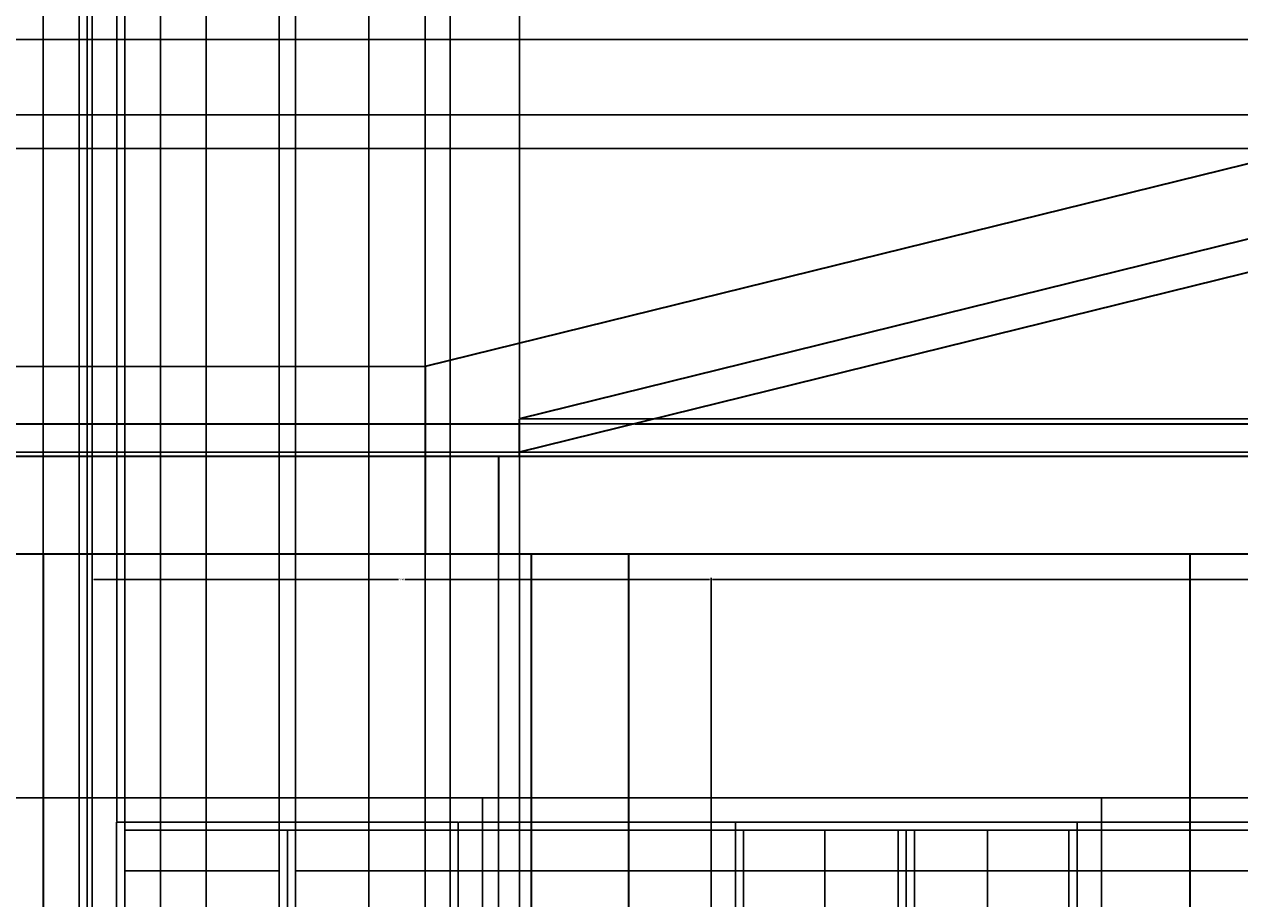
# Model space of a CAD drawing. Units: inches. Extents: x 2154 to 2740, y 571 to 1084.
# Tile 4 of 13: x 2235 to 2384, y 861 to 969. Entities that reach past the tile are written whole.
import ezdxf

# ---------------------------------------------------------------- set-up
doc = ezdxf.new("R2010")
doc.units = ezdxf.units.IN
for name, color, linetype, lineweight in [('A-ANNO-DIMS', 2, 'Continuous', 18), ('A-ELEV', 7, 'Continuous', 35), ('A-GLAZ', 4, 'Continuous', 25), ('A-ROOF', 1, 'Continuous', 35)]:
    doc.layers.add(name, color=color, linetype=linetype, lineweight=lineweight)
doc.styles.get("Standard").update_dxf_attribs({"font": 'arial.ttf'})
doc.dimstyles.get("Standard").update_dxf_attribs({"dimtxt": 0.18, "dimasz": 0.18, "dimexe": 0.18, "dimexo": 0.0625, "dimgap": 0.09, "dimtad": 0, "dimtih": 1, "dimtoh": 1, "dimdec": 4, "dimzin": 0, "dimdsep": 46, "dimtxsty": 'Standard', "dimcen": 0.09, "dimadec": 0, "dimazin": 0, "dimtfac": 1, "dimtdec": 4, "dimtofl": 0, "dimtmove": 0, "dimatfit": 3, "dimfxl": 1, "dimtolj": 1, "dimtzin": 0, "dimarcsym": 0})

# ---------------------------------------------------------------- blocks, each defined once
blk = doc.blocks.new('WIN-ELEV-1200')
for p, q in [((0, 50), (48, 50)), ((0, 0), (0, 50)), ((48, 0), (48, 50)), ((3, 0), (3, 47)), ((3, 47), (45, 47)), ((45, 0), (45, 47)), ((4, 46), (44, 46)), ((4, 0), (4, 46)), ((14, 0), (14, 46)), ((23, 0), (23, 46)), ((24, 0), (24, 46)), ((25, 0), (25, 46)), ((34, 0), (34, 46)), ((44, 0), (44, 46)), ((4, 41), (23, 41)), ((25, 41), (44, 41)), ((4, 32), (23, 32)), ((25, 32), (44, 32)), ((4, 23), (23, 23)), ((25, 23), (44, 23)), ((4, 14), (23, 14)), ((25, 14), (44, 14)), ((4, 5), (23, 5)), ((25, 5), (44, 5))]:
    blk.add_line(p, q)
blk = doc.blocks.new('*D8')
at = {"layer": 'A-ANNO-DIMS', "color": 0, "lineweight": -2, "transparency": 16777216}
for p, q in [((2284.21, 926.63), (2284.21, 953.59)), ((2601.21, 926.54), (2601.21, 953.51)), ((2284.39, 953.41), (2442.43, 953.37)), ((2601.03, 953.33), (2443, 953.37))]:
    blk.add_line(p, q, dxfattribs=at)
at = {"layer": 'A-ANNO-DIMS', "color": 0, "transparency": 16777216}
for points in [[(2284.39, 953.44), (2284.39, 953.38), (2284.21, 953.41)], [(2601.03, 953.36), (2601.03, 953.3), (2601.21, 953.33)]]:
    blk.add_solid(points, dxfattribs=at)
at = {"layer": 'Defpoints', "color": 0, "transparency": 16777216}
for p in [(2601.21, 953.33), (2284.21, 926.56), (2601.21, 926.48)]:
    blk.add_point(p, dxfattribs=at)
at = {"layer": 'A-ANNO-DIMS', "color": 0, "transparency": 16777216, "insert": (2442.71, 953.37), "char_height": 0.18, "attachment_point": 5}
blk.add_mtext('\\A1;317', dxfattribs=at)
blk = doc.blocks.new('*D10')
at = {"layer": 'A-ANNO-DIMS', "color": 0, "lineweight": -2, "transparency": 16777216}
for p, q in [((2447.14, 1057.01), (2154.18, 1057.01)), ((2154.36, 1056.83), (2154.36, 827.45)), ((2154.36, 597.71), (2154.36, 827.09)), ((2181.14, 597.53), (2154.18, 597.53))]:
    blk.add_line(p, q, dxfattribs=at)
at = {"layer": 'A-ANNO-DIMS', "color": 0, "transparency": 16777216}
for points in [[(2154.33, 1056.83), (2154.39, 1056.83), (2154.36, 1057.01)], [(2154.33, 597.71), (2154.39, 597.71), (2154.36, 597.53)]]:
    blk.add_solid(points, dxfattribs=at)
at = {"layer": 'Defpoints', "color": 0, "transparency": 16777216}
for p in [(2154.36, 1057.01), (2447.21, 1057.01), (2181.21, 597.53)]:
    blk.add_point(p, dxfattribs=at)
at = {"layer": 'A-ANNO-DIMS', "color": 0, "transparency": 16777216, "insert": (2154.36, 827.27), "char_height": 0.18, "attachment_point": 5}
blk.add_mtext('\\A1;459.5', dxfattribs=at)
blk = doc.blocks.new('*D33')
at = {"layer": 'A-ANNO-DIMS', "color": 0, "lineweight": -2, "transparency": 16777216}
for p, q in [((2412.64, 873.53), (2154.18, 873.53)), ((2154.36, 873.35), (2154.36, 848.71)), ((2154.36, 823.71), (2154.36, 848.35)), ((2412.64, 823.53), (2154.18, 823.53))]:
    blk.add_line(p, q, dxfattribs=at)
at = {"layer": 'A-ANNO-DIMS', "color": 0, "transparency": 16777216}
for points in [[(2154.33, 873.35), (2154.39, 873.35), (2154.36, 873.53)], [(2154.33, 823.71), (2154.39, 823.71), (2154.36, 823.53)]]:
    blk.add_solid(points, dxfattribs=at)
at = {"layer": 'Defpoints', "color": 0, "transparency": 16777216}
for p in [(2154.36, 873.53), (2412.71, 873.53), (2412.71, 823.53)]:
    blk.add_point(p, dxfattribs=at)
at = {"layer": 'A-ANNO-DIMS', "color": 0, "transparency": 16777216, "insert": (2154.36, 848.53), "char_height": 0.18, "attachment_point": 5}
blk.add_mtext('\\A1;50', dxfattribs=at)
blk = doc.blocks.new('*D35')
at = {"layer": 'A-ANNO-DIMS', "color": 0, "lineweight": -2, "transparency": 16777216}
for p, q in [((2447.21, 966.82), (2154.18, 966.82)), ((2154.36, 966.64), (2154.36, 946.87)), ((2154.36, 926.74), (2154.36, 946.51)), ((2284.14, 926.56), (2154.18, 926.56))]:
    blk.add_line(p, q, dxfattribs=at)
at = {"layer": 'A-ANNO-DIMS', "color": 0, "transparency": 16777216}
for points in [[(2154.33, 966.64), (2154.39, 966.64), (2154.36, 966.82)], [(2154.33, 926.74), (2154.39, 926.74), (2154.36, 926.56)]]:
    blk.add_solid(points, dxfattribs=at)
at = {"layer": 'Defpoints', "color": 0, "transparency": 16777216}
for p in [(2154.36, 966.82), (2447.27, 966.82), (2284.21, 926.56)]:
    blk.add_point(p, dxfattribs=at)
at = {"layer": 'A-ANNO-DIMS', "color": 0, "transparency": 16777216, "insert": (2154.36, 946.69), "char_height": 0.18, "attachment_point": 5}
blk.add_mtext('\\A1;40.255', dxfattribs=at)
blk = doc.blocks.new('*D36')
at = {"layer": 'A-ANNO-DIMS', "color": 0, "lineweight": -2, "transparency": 16777216}
for p, q in [((2447.21, 966.82), (2154.18, 966.82)), ((2154.36, 966.64), (2154.36, 962.36)), ((2154.36, 957.71), (2154.36, 961.99)), ((2447.14, 957.53), (2154.18, 957.53))]:
    blk.add_line(p, q, dxfattribs=at)
at = {"layer": 'A-ANNO-DIMS', "color": 0, "transparency": 16777216}
for points in [[(2154.33, 966.64), (2154.39, 966.64), (2154.36, 966.82)], [(2154.33, 957.71), (2154.39, 957.71), (2154.36, 957.53)]]:
    blk.add_solid(points, dxfattribs=at)
at = {"layer": 'Defpoints', "color": 0, "transparency": 16777216}
for p in [(2154.36, 966.82), (2447.27, 966.82), (2447.21, 957.53)]:
    blk.add_point(p, dxfattribs=at)
at = {"layer": 'A-ANNO-DIMS', "color": 0, "transparency": 16777216, "insert": (2154.36, 962.18), "char_height": 0.18, "attachment_point": 5}
blk.add_mtext('\\A1;9.287', dxfattribs=at)
blk = doc.blocks.new('*D37')
at = {"layer": 'A-ANNO-DIMS', "color": 0, "lineweight": -2, "transparency": 16777216}
for p, q in [((2447.14, 957.53), (2154.18, 957.53)), ((2154.36, 957.35), (2154.36, 955.65)), ((2154.36, 953.58), (2154.36, 955.29)), ((2447.11, 953.4), (2154.18, 953.4))]:
    blk.add_line(p, q, dxfattribs=at)
at = {"layer": 'A-ANNO-DIMS', "color": 0, "transparency": 16777216}
for points in [[(2154.33, 957.35), (2154.39, 957.35), (2154.36, 957.53)], [(2154.33, 953.58), (2154.39, 953.58), (2154.36, 953.4)]]:
    blk.add_solid(points, dxfattribs=at)
at = {"layer": 'Defpoints', "color": 0, "transparency": 16777216}
for p in [(2154.36, 957.53), (2447.21, 957.53), (2447.18, 953.4)]:
    blk.add_point(p, dxfattribs=at)
at = {"layer": 'A-ANNO-DIMS', "color": 0, "transparency": 16777216, "insert": (2154.36, 955.47), "char_height": 0.18, "attachment_point": 5}
blk.add_mtext('\\A1;4.127', dxfattribs=at)
blk = doc.blocks.new('*D38')
at = {"layer": 'A-ANNO-DIMS', "color": 0, "lineweight": -2, "transparency": 16777216}
for p, q in [((2447.11, 953.4), (2154.18, 953.4)), ((2154.36, 953.22), (2154.36, 934.9)), ((2154.36, 916.21), (2154.36, 934.53)), ((2295.71, 916.03), (2154.18, 916.03))]:
    blk.add_line(p, q, dxfattribs=at)
at = {"layer": 'A-ANNO-DIMS', "color": 0, "transparency": 16777216}
for points in [[(2154.33, 953.22), (2154.39, 953.22), (2154.36, 953.4)], [(2154.33, 916.21), (2154.39, 916.21), (2154.36, 916.03)]]:
    blk.add_solid(points, dxfattribs=at)
at = {"layer": 'Defpoints', "color": 0, "transparency": 16777216}
for p in [(2154.36, 953.4), (2447.18, 953.4), (2295.77, 916.03)]:
    blk.add_point(p, dxfattribs=at)
at = {"layer": 'A-ANNO-DIMS', "color": 0, "transparency": 16777216, "insert": (2154.36, 934.72), "char_height": 0.18, "attachment_point": 5}
blk.add_mtext('\\A1;37.38', dxfattribs=at)
blk = doc.blocks.new('*D39')
at = {"layer": 'A-ANNO-DIMS', "color": 0, "lineweight": -2, "transparency": 16777216}
for p, q in [((2183.21, 979.47), (2183.21, 570.5)), ((2417.21, 970.47), (2417.21, 570.5)), ((2183.39, 570.68), (2299.92, 570.68)), ((2417.03, 570.68), (2300.5, 570.68))]:
    blk.add_line(p, q, dxfattribs=at)
at = {"layer": 'A-ANNO-DIMS', "color": 0, "transparency": 16777216}
for points in [[(2183.39, 570.71), (2183.39, 570.65), (2183.21, 570.68)], [(2417.03, 570.71), (2417.03, 570.65), (2417.21, 570.68)]]:
    blk.add_solid(points, dxfattribs=at)
at = {"layer": 'Defpoints', "color": 0, "transparency": 16777216}
for p in [(2183.21, 979.53), (2417.21, 970.53), (2417.21, 570.68)]:
    blk.add_point(p, dxfattribs=at)
at = {"layer": 'A-ANNO-DIMS', "color": 0, "transparency": 16777216, "insert": (2300.21, 570.68), "char_height": 0.18, "attachment_point": 5}
blk.add_mtext('\\A1;234', dxfattribs=at)
blk = doc.blocks.new('*D40')
at = {"layer": 'A-ANNO-DIMS', "color": 0, "lineweight": -2, "transparency": 16777216}
for p, q in [((2243.26, 873.59), (2243.26, 900.56)), ((2243.44, 900.38), (2280.91, 900.38)), ((2319.17, 900.38), (2281.7, 900.38)), ((2319.35, 873.59), (2319.35, 900.56))]:
    blk.add_line(p, q, dxfattribs=at)
at = {"layer": 'A-ANNO-DIMS', "color": 0, "transparency": 16777216}
for points in [[(2243.44, 900.41), (2243.44, 900.35), (2243.26, 900.38)], [(2319.17, 900.41), (2319.17, 900.35), (2319.35, 900.38)]]:
    blk.add_solid(points, dxfattribs=at)
at = {"layer": 'Defpoints', "color": 0, "transparency": 16777216}
for p in [(2319.35, 900.38), (2243.26, 873.53), (2319.35, 873.53)]:
    blk.add_point(p, dxfattribs=at)
at = {"layer": 'A-ANNO-DIMS', "color": 0, "transparency": 16777216, "insert": (2281.3, 900.38), "char_height": 0.18, "attachment_point": 5}
blk.add_mtext('\\A1;76.09', dxfattribs=at)
blk = doc.blocks.new('*D41')
at = {"layer": 'A-ANNO-DIMS', "color": 0, "lineweight": -2, "transparency": 16777216}
for p, q in [((2319.35, 873.59), (2319.35, 900.56)), ((2319.53, 900.38), (2418.06, 900.38)), ((2517.5, 900.38), (2418.97, 900.38)), ((2517.68, 873.59), (2517.68, 900.56))]:
    blk.add_line(p, q, dxfattribs=at)
at = {"layer": 'A-ANNO-DIMS', "color": 0, "transparency": 16777216}
for points in [[(2319.53, 900.41), (2319.53, 900.35), (2319.35, 900.38)], [(2517.5, 900.41), (2517.5, 900.35), (2517.68, 900.38)]]:
    blk.add_solid(points, dxfattribs=at)
at = {"layer": 'Defpoints', "color": 0, "transparency": 16777216}
for p in [(2517.68, 900.38), (2319.35, 873.53), (2517.68, 873.53)]:
    blk.add_point(p, dxfattribs=at)
at = {"layer": 'A-ANNO-DIMS', "color": 0, "transparency": 16777216, "insert": (2418.51, 900.38), "char_height": 0.18, "attachment_point": 5}
blk.add_mtext('\\A1;198.33', dxfattribs=at)
blk = doc.blocks.new('*D46')
at = {"layer": 'A-ANNO-DIMS', "color": 0, "lineweight": -2, "transparency": 16777216}
for p, q in [((2195.27, 915.53), (2740.24, 915.53)), ((2740.06, 915.35), (2740.06, 909.71)), ((2740.06, 903.71), (2740.06, 909.35)), ((2195.27, 903.53), (2740.24, 903.53))]:
    blk.add_line(p, q, dxfattribs=at)
at = {"layer": 'A-ANNO-DIMS', "color": 0, "transparency": 16777216}
for points in [[(2740.03, 915.35), (2740.09, 915.35), (2740.06, 915.53)], [(2740.03, 903.71), (2740.09, 903.71), (2740.06, 903.53)]]:
    blk.add_solid(points, dxfattribs=at)
at = {"layer": 'Defpoints', "color": 0, "transparency": 16777216}
for p in [(2195.21, 915.53), (2740.06, 915.53), (2195.21, 903.53)]:
    blk.add_point(p, dxfattribs=at)
at = {"layer": 'A-ANNO-DIMS', "color": 0, "transparency": 16777216, "insert": (2740.06, 909.53), "char_height": 0.18, "attachment_point": 5}
blk.add_mtext('\\A1;12', dxfattribs=at)
blk = doc.blocks.new('*D47')
at = {"layer": 'A-ANNO-DIMS', "color": 0, "lineweight": -2, "transparency": 16777216}
for p, q in [((2195.269199, 919.532069), (2740.236699, 919.532069)), ((2740.056699, 919.352069), (2740.056699, 917.712069)), ((2740.056699, 915.712069), (2740.056699, 917.352069)), ((2195.269199, 915.532069), (2740.236699, 915.532069))]:
    blk.add_line(p, q, dxfattribs=at)
at = {"layer": 'A-ANNO-DIMS', "color": 0, "transparency": 16777216}
for points in [[(2740.026699, 919.352069), (2740.086699, 919.352069), (2740.056699, 919.532069)], [(2740.026699, 915.712069), (2740.086699, 915.712069), (2740.056699, 915.532069)]]:
    blk.add_solid(points, dxfattribs=at)
at = {"layer": 'Defpoints', "color": 0, "transparency": 16777216}
for p in [(2195.206699, 919.532069), (2740.056699, 919.532069), (2195.206699, 915.532069)]:
    blk.add_point(p, dxfattribs=at)
at = {"layer": 'A-ANNO-DIMS', "color": 0, "transparency": 16777216, "insert": (2740.056699, 917.532069), "char_height": 0.18, "attachment_point": 5}
blk.add_mtext('\\A1;4', dxfattribs=at)
blk = doc.blocks.new('*D48')
at = {"layer": 'A-ANNO-DIMS', "color": 0, "lineweight": -2, "transparency": 16777216}
for p, q in [((2195.27, 979.53), (2740.24, 979.53)), ((2740.06, 979.35), (2740.06, 949.71)), ((2740.06, 919.71), (2740.06, 949.35)), ((2195.27, 919.53), (2740.24, 919.53))]:
    blk.add_line(p, q, dxfattribs=at)
at = {"layer": 'A-ANNO-DIMS', "color": 0, "transparency": 16777216}
for points in [[(2740.03, 979.35), (2740.09, 979.35), (2740.06, 979.53)], [(2740.03, 919.71), (2740.09, 919.71), (2740.06, 919.53)]]:
    blk.add_solid(points, dxfattribs=at)
at = {"layer": 'Defpoints', "color": 0, "transparency": 16777216}
for p in [(2195.21, 979.53), (2740.06, 979.53), (2195.21, 919.53)]:
    blk.add_point(p, dxfattribs=at)
at = {"layer": 'A-ANNO-DIMS', "color": 0, "transparency": 16777216, "insert": (2740.06, 949.53), "char_height": 0.18, "attachment_point": 5}
blk.add_mtext('\\A1;60', dxfattribs=at)
blk = doc.blocks.new('*D52')
at = {"layer": 'A-ANNO-DIMS', "color": 0, "lineweight": -2, "transparency": 16777216}
for p, q in [((2284.21, 903.47), (2284.21, 570.5)), ((2293.21, 903.47), (2293.21, 570.5)), ((2284.39, 570.68), (2288.56, 570.68)), ((2293.03, 570.68), (2288.86, 570.68))]:
    blk.add_line(p, q, dxfattribs=at)
at = {"layer": 'A-ANNO-DIMS', "color": 0, "transparency": 16777216}
for points in [[(2284.39, 570.71), (2284.39, 570.65), (2284.21, 570.68)], [(2293.03, 570.71), (2293.03, 570.65), (2293.21, 570.68)]]:
    blk.add_solid(points, dxfattribs=at)
at = {"layer": 'Defpoints', "color": 0, "transparency": 16777216}
for p in [(2284.21, 903.53), (2293.21, 903.53), (2293.21, 570.68)]:
    blk.add_point(p, dxfattribs=at)
at = {"layer": 'A-ANNO-DIMS', "color": 0, "transparency": 16777216, "insert": (2288.71, 570.68), "char_height": 0.18, "attachment_point": 5}
blk.add_mtext('\\A1;9', dxfattribs=at)
blk = doc.blocks.new('*D53')
at = {"layer": 'A-ANNO-DIMS', "color": 0, "lineweight": -2, "transparency": 16777216}
for p, q in [((2284.21, 926.63), (2284.21, 1084.04)), ((2284.39, 1083.86), (2289.53, 1083.86)), ((2295.59, 1083.86), (2290.45, 1083.86)), ((2295.77, 920.21), (2295.77, 1084.04))]:
    blk.add_line(p, q, dxfattribs=at)
at = {"layer": 'A-ANNO-DIMS', "color": 0, "transparency": 16777216}
for points in [[(2284.39, 1083.89), (2284.39, 1083.83), (2284.21, 1083.86)], [(2295.59, 1083.89), (2295.59, 1083.83), (2295.77, 1083.86)]]:
    blk.add_solid(points, dxfattribs=at)
at = {"layer": 'Defpoints', "color": 0, "transparency": 16777216}
for p in [(2295.77, 1083.86), (2284.21, 926.56), (2295.77, 920.15)]:
    blk.add_point(p, dxfattribs=at)
at = {"layer": 'A-ANNO-DIMS', "color": 0, "transparency": 16777216, "insert": (2289.99, 1083.86), "char_height": 0.18, "attachment_point": 5}
blk.add_mtext('\\A1;11.566', dxfattribs=at)
blk = doc.blocks.new('*D54')
at = {"layer": 'A-ANNO-DIMS', "color": 0, "lineweight": -2, "transparency": 16777216}
for p, q in [((2284.14, 926.56), (2154.18, 926.56)), ((2154.36, 926.38), (2154.36, 915.23)), ((2154.36, 903.71), (2154.36, 914.87)), ((2284.14, 903.53), (2154.18, 903.53))]:
    blk.add_line(p, q, dxfattribs=at)
at = {"layer": 'A-ANNO-DIMS', "color": 0, "transparency": 16777216}
for points in [[(2154.33, 926.38), (2154.39, 926.38), (2154.36, 926.56)], [(2154.33, 903.71), (2154.39, 903.71), (2154.36, 903.53)]]:
    blk.add_solid(points, dxfattribs=at)
at = {"layer": 'Defpoints', "color": 0, "transparency": 16777216}
for p in [(2154.36, 926.56), (2284.21, 926.56), (2284.21, 903.53)]:
    blk.add_point(p, dxfattribs=at)
at = {"layer": 'A-ANNO-DIMS', "color": 0, "transparency": 16777216, "insert": (2154.36, 915.05), "char_height": 0.18, "attachment_point": 5}
blk.add_mtext('\\A1;23.03', dxfattribs=at)
blk = doc.blocks.new('*D55')
at = {"layer": 'A-ANNO-DIMS', "color": 0, "lineweight": -2, "transparency": 16777216}
for p, q in [((2295.84, 920.15), (2740.24, 920.15)), ((2740.06, 919.97), (2740.06, 918.27)), ((2740.06, 916.21), (2740.06, 917.91)), ((2295.83, 916.03), (2740.24, 916.03))]:
    blk.add_line(p, q, dxfattribs=at)
at = {"layer": 'A-ANNO-DIMS', "color": 0, "transparency": 16777216}
for points in [[(2740.03, 919.97), (2740.09, 919.97), (2740.06, 920.15)], [(2740.03, 916.21), (2740.09, 916.21), (2740.06, 916.03)]]:
    blk.add_solid(points, dxfattribs=at)
at = {"layer": 'Defpoints', "color": 0, "transparency": 16777216}
for p in [(2295.77, 920.15), (2740.06, 920.15), (2295.77, 916.03)]:
    blk.add_point(p, dxfattribs=at)
at = {"layer": 'A-ANNO-DIMS', "color": 0, "transparency": 16777216, "insert": (2740.06, 918.09), "char_height": 0.18, "attachment_point": 5}
blk.add_mtext('\\A1;4.12', dxfattribs=at)
blk = doc.blocks.new('*D56')
at = {"layer": 'A-ANNO-DIMS', "color": 0, "lineweight": -2, "transparency": 16777216}
for p, q in [((2293.21, 915.47), (2293.21, 570.5)), ((2295.77, 915.97), (2295.77, 570.5)), ((2293.39, 570.68), (2294.16, 570.68)), ((2295.59, 570.68), (2294.81, 570.68))]:
    blk.add_line(p, q, dxfattribs=at)
at = {"layer": 'A-ANNO-DIMS', "color": 0, "transparency": 16777216}
for points in [[(2293.39, 570.71), (2293.39, 570.65), (2293.21, 570.68)], [(2295.59, 570.71), (2295.59, 570.65), (2295.77, 570.68)]]:
    blk.add_solid(points, dxfattribs=at)
at = {"layer": 'Defpoints', "color": 0, "transparency": 16777216}
for p in [(2293.21, 915.53), (2295.77, 916.03), (2295.77, 570.68)]:
    blk.add_point(p, dxfattribs=at)
at = {"layer": 'A-ANNO-DIMS', "color": 0, "transparency": 16777216, "insert": (2294.49, 570.68), "char_height": 0.18, "attachment_point": 5}
blk.add_mtext('\\A1;2.56', dxfattribs=at)
blk = doc.blocks.new('*D65')
at = {"layer": 'A-ANNO-DIMS', "color": 0, "lineweight": -2, "transparency": 16777216}
for p, q in [((2225.21, 777.59), (2225.21, 1084.04)), ((2225.39, 1083.86), (2231, 1083.86)), ((2237.03, 1083.86), (2231.42, 1083.86)), ((2237.21, 777.59), (2237.21, 1084.04))]:
    blk.add_line(p, q, dxfattribs=at)
at = {"layer": 'A-ANNO-DIMS', "color": 0, "transparency": 16777216}
for points in [[(2225.39, 1083.89), (2225.39, 1083.83), (2225.21, 1083.86)], [(2237.03, 1083.89), (2237.03, 1083.83), (2237.21, 1083.86)]]:
    blk.add_solid(points, dxfattribs=at)
at = {"layer": 'Defpoints', "color": 0, "transparency": 16777216}
for p in [(2237.21, 1083.86), (2225.21, 777.53), (2237.21, 777.53)]:
    blk.add_point(p, dxfattribs=at)
at = {"layer": 'A-ANNO-DIMS', "color": 0, "transparency": 16777216, "insert": (2231.21, 1083.86), "char_height": 0.18, "attachment_point": 5}
blk.add_mtext('\\A1;12', dxfattribs=at)
blk = doc.blocks.new('*D110')
at = {"layer": 'A-ANNO-DIMS', "color": 0, "lineweight": -2, "transparency": 16777216}
for p, q in [((2237.21, 823.59), (2237.21, 1084.04)), ((2237.39, 1083.86), (2239.91, 1083.86)), ((2243.08, 1083.86), (2240.56, 1083.86)), ((2243.26, 823.59), (2243.26, 1084.04))]:
    blk.add_line(p, q, dxfattribs=at)
at = {"layer": 'A-ANNO-DIMS', "color": 0, "transparency": 16777216}
for points in [[(2237.39, 1083.89), (2237.39, 1083.83), (2237.21, 1083.86)], [(2243.08, 1083.89), (2243.08, 1083.83), (2243.26, 1083.86)]]:
    blk.add_solid(points, dxfattribs=at)
at = {"layer": 'Defpoints', "color": 0, "transparency": 16777216}
for p in [(2243.26, 1083.86), (2237.21, 823.53), (2243.26, 823.53)]:
    blk.add_point(p, dxfattribs=at)
at = {"layer": 'A-ANNO-DIMS', "color": 0, "transparency": 16777216, "insert": (2240.23, 1083.86), "char_height": 0.18, "attachment_point": 5}
blk.add_mtext('\\A1;6.05', dxfattribs=at)
blk = doc.blocks.new('*D111')
at = {"layer": 'A-ANNO-DIMS', "color": 0, "lineweight": -2, "transparency": 16777216}
for p, q in [((2243.26, 873.59), (2243.26, 1084.04)), ((2243.44, 1083.86), (2244.61, 1083.86)), ((2246.08, 1083.86), (2244.91, 1083.86)), ((2246.26, 870.59), (2246.26, 1084.04))]:
    blk.add_line(p, q, dxfattribs=at)
at = {"layer": 'A-ANNO-DIMS', "color": 0, "transparency": 16777216}
for points in [[(2243.44, 1083.89), (2243.44, 1083.83), (2243.26, 1083.86)], [(2246.08, 1083.89), (2246.08, 1083.83), (2246.26, 1083.86)]]:
    blk.add_solid(points, dxfattribs=at)
at = {"layer": 'Defpoints', "color": 0, "transparency": 16777216}
for p in [(2246.26, 1083.86), (2243.26, 873.53), (2246.26, 870.53)]:
    blk.add_point(p, dxfattribs=at)
at = {"layer": 'A-ANNO-DIMS', "color": 0, "transparency": 16777216, "insert": (2244.76, 1083.86), "char_height": 0.18, "attachment_point": 5}
blk.add_mtext('\\A1;3', dxfattribs=at)
blk = doc.blocks.new('*D112')
at = {"layer": 'A-ANNO-DIMS', "color": 0, "lineweight": -2, "transparency": 16777216}
for p, q in [((2291.32, 873.53), (2740.24, 873.53)), ((2740.06, 873.35), (2740.06, 872.21)), ((2740.06, 870.71), (2740.06, 871.85)), ((2288.32, 870.53), (2740.24, 870.53))]:
    blk.add_line(p, q, dxfattribs=at)
at = {"layer": 'A-ANNO-DIMS', "color": 0, "transparency": 16777216}
for points in [[(2740.03, 873.35), (2740.09, 873.35), (2740.06, 873.53)], [(2740.03, 870.71), (2740.09, 870.71), (2740.06, 870.53)]]:
    blk.add_solid(points, dxfattribs=at)
at = {"layer": 'Defpoints', "color": 0, "transparency": 16777216}
for p in [(2291.26, 873.53), (2740.06, 873.53), (2288.26, 870.53)]:
    blk.add_point(p, dxfattribs=at)
at = {"layer": 'A-ANNO-DIMS', "color": 0, "transparency": 16777216, "insert": (2740.06, 872.03), "char_height": 0.18, "attachment_point": 5}
blk.add_mtext('\\A1;3', dxfattribs=at)
blk = doc.blocks.new('*D113')
at = {"layer": 'A-ANNO-DIMS', "color": 0, "lineweight": -2, "transparency": 16777216}
for p, q in [((2246.26, 870.59), (2246.26, 1084.04)), ((2246.44, 1083.86), (2246.63, 1083.86)), ((2247.08, 1083.86), (2246.88, 1083.86)), ((2247.26, 869.59), (2247.26, 1084.04))]:
    blk.add_line(p, q, dxfattribs=at)
at = {"layer": 'A-ANNO-DIMS', "color": 0, "transparency": 16777216}
for points in [[(2246.44, 1083.89), (2246.44, 1083.83), (2246.26, 1083.86)], [(2247.08, 1083.89), (2247.08, 1083.83), (2247.26, 1083.86)]]:
    blk.add_solid(points, dxfattribs=at)
at = {"layer": 'Defpoints', "color": 0, "transparency": 16777216}
for p in [(2247.26, 1083.86), (2246.26, 870.53), (2247.26, 869.53)]:
    blk.add_point(p, dxfattribs=at)
at = {"layer": 'A-ANNO-DIMS', "color": 0, "transparency": 16777216, "insert": (2246.76, 1083.86), "char_height": 0.18, "attachment_point": 5}
blk.add_mtext('\\A1;1', dxfattribs=at)
blk = doc.blocks.new('*D114')
at = {"layer": 'A-ANNO-DIMS', "color": 0, "lineweight": -2, "transparency": 16777216}
for p, q in [((2247.26, 869.59), (2247.26, 1084.04)), ((2247.44, 1083.86), (2252.05, 1083.86)), ((2257.08, 1083.86), (2252.47, 1083.86)), ((2257.26, 869.59), (2257.26, 1084.04))]:
    blk.add_line(p, q, dxfattribs=at)
at = {"layer": 'A-ANNO-DIMS', "color": 0, "transparency": 16777216}
for points in [[(2247.44, 1083.89), (2247.44, 1083.83), (2247.26, 1083.86)], [(2257.08, 1083.89), (2257.08, 1083.83), (2257.26, 1083.86)]]:
    blk.add_solid(points, dxfattribs=at)
at = {"layer": 'Defpoints', "color": 0, "transparency": 16777216}
for p in [(2257.26, 1083.86), (2247.26, 869.53), (2257.26, 869.53)]:
    blk.add_point(p, dxfattribs=at)
at = {"layer": 'A-ANNO-DIMS', "color": 0, "transparency": 16777216, "insert": (2252.26, 1083.86), "char_height": 0.18, "attachment_point": 5}
blk.add_mtext('\\A1;10', dxfattribs=at)
blk = doc.blocks.new('*D115')
at = {"layer": 'A-ANNO-DIMS', "color": 0, "lineweight": -2, "transparency": 16777216}
for p, q in [((2257.26, 869.59), (2257.26, 1084.04)), ((2257.44, 1083.86), (2261.61, 1083.86)), ((2266.08, 1083.86), (2261.91, 1083.86)), ((2266.26, 869.59), (2266.26, 1084.04))]:
    blk.add_line(p, q, dxfattribs=at)
at = {"layer": 'A-ANNO-DIMS', "color": 0, "transparency": 16777216}
for points in [[(2257.44, 1083.89), (2257.44, 1083.83), (2257.26, 1083.86)], [(2266.08, 1083.89), (2266.08, 1083.83), (2266.26, 1083.86)]]:
    blk.add_solid(points, dxfattribs=at)
at = {"layer": 'Defpoints', "color": 0, "transparency": 16777216}
for p in [(2266.26, 1083.86), (2257.26, 869.53), (2266.26, 869.53)]:
    blk.add_point(p, dxfattribs=at)
at = {"layer": 'A-ANNO-DIMS', "color": 0, "transparency": 16777216, "insert": (2261.76, 1083.86), "char_height": 0.18, "attachment_point": 5}
blk.add_mtext('\\A1;9', dxfattribs=at)
blk = doc.blocks.new('*D116')
at = {"layer": 'A-ANNO-DIMS', "color": 0, "lineweight": -2, "transparency": 16777216}
for p, q in [((2266.26, 869.59), (2266.26, 1084.04)), ((2266.44, 1083.86), (2267.11, 1083.86)), ((2268.08, 1083.86), (2267.41, 1083.86)), ((2268.26, 869.59), (2268.26, 1084.04))]:
    blk.add_line(p, q, dxfattribs=at)
at = {"layer": 'A-ANNO-DIMS', "color": 0, "transparency": 16777216}
for points in [[(2266.44, 1083.89), (2266.44, 1083.83), (2266.26, 1083.86)], [(2268.08, 1083.89), (2268.08, 1083.83), (2268.26, 1083.86)]]:
    blk.add_solid(points, dxfattribs=at)
at = {"layer": 'Defpoints', "color": 0, "transparency": 16777216}
for p in [(2268.26, 1083.86), (2266.26, 869.53), (2268.26, 869.53)]:
    blk.add_point(p, dxfattribs=at)
at = {"layer": 'A-ANNO-DIMS', "color": 0, "transparency": 16777216, "insert": (2267.26, 1083.86), "char_height": 0.18, "attachment_point": 5}
blk.add_mtext('\\A1;2', dxfattribs=at)
blk = doc.blocks.new('*D117')
at = {"layer": 'A-ANNO-DIMS', "color": 0, "lineweight": -2, "transparency": 16777216}
for p, q in [((2268.26, 869.59), (2268.26, 1084.04)), ((2268.44, 1083.86), (2272.61, 1083.86)), ((2277.08, 1083.86), (2272.91, 1083.86)), ((2277.26, 869.59), (2277.26, 1084.04))]:
    blk.add_line(p, q, dxfattribs=at)
at = {"layer": 'A-ANNO-DIMS', "color": 0, "transparency": 16777216}
for points in [[(2268.44, 1083.89), (2268.44, 1083.83), (2268.26, 1083.86)], [(2277.08, 1083.89), (2277.08, 1083.83), (2277.26, 1083.86)]]:
    blk.add_solid(points, dxfattribs=at)
at = {"layer": 'Defpoints', "color": 0, "transparency": 16777216}
for p in [(2277.26, 1083.86), (2268.26, 869.53), (2277.26, 869.53)]:
    blk.add_point(p, dxfattribs=at)
at = {"layer": 'A-ANNO-DIMS', "color": 0, "transparency": 16777216, "insert": (2272.76, 1083.86), "char_height": 0.18, "attachment_point": 5}
blk.add_mtext('\\A1;9', dxfattribs=at)
blk = doc.blocks.new('*D118')
at = {"layer": 'A-ANNO-DIMS', "color": 0, "lineweight": -2, "transparency": 16777216}
for p, q in [((2277.26, 869.59), (2277.26, 1084.04)), ((2277.44, 1083.86), (2282.05, 1083.86)), ((2287.08, 1083.86), (2282.47, 1083.86)), ((2287.26, 869.59), (2287.26, 1084.04))]:
    blk.add_line(p, q, dxfattribs=at)
at = {"layer": 'A-ANNO-DIMS', "color": 0, "transparency": 16777216}
for points in [[(2277.44, 1083.89), (2277.44, 1083.83), (2277.26, 1083.86)], [(2287.08, 1083.89), (2287.08, 1083.83), (2287.26, 1083.86)]]:
    blk.add_solid(points, dxfattribs=at)
at = {"layer": 'Defpoints', "color": 0, "transparency": 16777216}
for p in [(2287.26, 1083.86), (2277.26, 869.53), (2287.26, 869.53)]:
    blk.add_point(p, dxfattribs=at)
at = {"layer": 'A-ANNO-DIMS', "color": 0, "transparency": 16777216, "insert": (2282.26, 1083.86), "char_height": 0.18, "attachment_point": 5}
blk.add_mtext('\\A1;10', dxfattribs=at)
blk = doc.blocks.new('*D121')
at = {"layer": 'A-ANNO-DIMS', "color": 0, "lineweight": -2, "transparency": 16777216}
for p, q in [((2287.32, 869.53), (2740.24, 869.53)), ((2740.06, 869.35), (2740.06, 867.21)), ((2740.06, 864.71), (2740.06, 866.85)), ((2287.32, 864.53), (2740.24, 864.53))]:
    blk.add_line(p, q, dxfattribs=at)
at = {"layer": 'A-ANNO-DIMS', "color": 0, "transparency": 16777216}
for points in [[(2740.03, 869.35), (2740.09, 869.35), (2740.06, 869.53)], [(2740.03, 864.71), (2740.09, 864.71), (2740.06, 864.53)]]:
    blk.add_solid(points, dxfattribs=at)
at = {"layer": 'Defpoints', "color": 0, "transparency": 16777216}
for p in [(2287.26, 869.53), (2740.06, 869.53), (2287.26, 864.53)]:
    blk.add_point(p, dxfattribs=at)
at = {"layer": 'A-ANNO-DIMS', "color": 0, "transparency": 16777216, "insert": (2740.06, 867.03), "char_height": 0.18, "attachment_point": 5}
blk.add_mtext('\\A1;5', dxfattribs=at)
blk = doc.blocks.new('*D136')
at = {"layer": 'A-ANNO-DIMS', "color": 0, "lineweight": -2, "transparency": 16777216}
for p, q in [((2241.65, 648.59), (2241.65, 1084.04)), ((2241.83, 1083.86), (2242.03, 1083.86)), ((2242.47, 1083.86), (2242.28, 1083.86)), ((2242.65, 648.59), (2242.65, 1084.04))]:
    blk.add_line(p, q, dxfattribs=at)
at = {"layer": 'A-ANNO-DIMS', "color": 0, "transparency": 16777216}
for points in [[(2241.83, 1083.89), (2241.83, 1083.83), (2241.65, 1083.86)], [(2242.47, 1083.89), (2242.47, 1083.83), (2242.65, 1083.86)]]:
    blk.add_solid(points, dxfattribs=at)
at = {"layer": 'Defpoints', "color": 0, "transparency": 16777216}
for p in [(2242.65, 1083.86), (2241.65, 648.53), (2242.65, 648.53)]:
    blk.add_point(p, dxfattribs=at)
at = {"layer": 'A-ANNO-DIMS', "color": 0, "transparency": 16777216, "insert": (2242.15, 1083.86), "char_height": 0.18, "attachment_point": 5}
blk.add_mtext('\\A1;1', dxfattribs=at)
blk = doc.blocks.new('*D137')
at = {"layer": 'A-ANNO-DIMS', "color": 0, "lineweight": -2, "transparency": 16777216}
for p, q in [((2242.65, 648.59), (2242.65, 1084.04)), ((2242.83, 1083.86), (2247, 1083.86)), ((2251.47, 1083.86), (2247.3, 1083.86)), ((2251.65, 648.59), (2251.65, 1084.04))]:
    blk.add_line(p, q, dxfattribs=at)
at = {"layer": 'A-ANNO-DIMS', "color": 0, "transparency": 16777216}
for points in [[(2242.83, 1083.89), (2242.83, 1083.83), (2242.65, 1083.86)], [(2251.47, 1083.89), (2251.47, 1083.83), (2251.65, 1083.86)]]:
    blk.add_solid(points, dxfattribs=at)
at = {"layer": 'Defpoints', "color": 0, "transparency": 16777216}
for p in [(2251.65, 1083.86), (2242.65, 648.53), (2251.65, 648.53)]:
    blk.add_point(p, dxfattribs=at)
at = {"layer": 'A-ANNO-DIMS', "color": 0, "transparency": 16777216, "insert": (2247.15, 1083.86), "char_height": 0.18, "attachment_point": 5}
blk.add_mtext('\\A1;9', dxfattribs=at)

msp = doc.modelspace()

# ---------------------------------------------------------------- linework, layer by layer
at = {"layer": 'A-ELEV'}
for p, q in [((2237.2067, 903.5321), (2237.2067, 777.5321)), ((2297.2067, 903.5321), (2297.2067, 777.5321)), ((2309.2067, 903.5321), (2309.2067, 777.5321)), ((2378.2067, 903.5321), (2378.2067, 777.5321))]:
    msp.add_line(p, q, dxfattribs=at)
at = {"layer": 'A-ROOF'}
for p, q in [((2447.273, 966.8186), (2284.2067, 926.5633)), ((2447.2067, 957.5321), (2295.7731, 920.1485)), ((2447.1772, 953.4047), (2295.7714, 916.028)), ((2284.2067, 926.5633), (2284.2067, 903.5321)), ((2195.2067, 919.5321), (2295.7729, 919.5321)), ((2295.7712, 915.5321), (2295.7731, 920.1485)), ((2309.9659, 919.5321), (2576.4281, 919.5321)), ((2195.2067, 915.5321), (2699.2067, 915.5321)), ((2293.2067, 915.5321), (2293.2067, 903.5321)), ((2195.2067, 903.5321), (2699.2067, 903.5321))]:
    msp.add_line(p, q, dxfattribs=at)

# ---------------------------------------------------------------- block references
at = {"layer": 'A-GLAZ'}
for p in [(2243.2571, 823.532), (2319.3479, 823.532)]:
    msp.add_blockref('WIN-ELEV-1200', p, dxfattribs=at)

# ---------------------------------------------------------------- dimensions: what is measured, and where the dimension line sits
at = {"layer": 'A-ANNO-DIMS'}
for base, p1, p2, override, picture, middle in [((2237.2067, 1083.8553), (2225.2067, 777.5321), (2237.2067, 777.5321), {"dimdec": 0, "dimlfac": 1, "dimrnd": 0, "dimzin": 0, "dimdsep": 46, "dimlunit": 2}, '*D65', (2231.2067, 1083.8553)), ((2243.2568, 1083.8553), (2237.2067, 823.5321), (2243.2568, 823.5321), {"dimdec": 2, "dimlfac": 1, "dimrnd": 0, "dimzin": 0, "dimdsep": 46, "dimlunit": 2}, '*D110', (2240.2317, 1083.8553)), ((2242.6527, 1083.8553), (2241.6527, 648.5321), (2242.6527, 648.5321), {"dimdec": 0, "dimlfac": 1, "dimrnd": 0, "dimzin": 0, "dimdsep": 46, "dimlunit": 2}, '*D136', (2242.1527, 1083.8553)), ((2251.6527, 1083.8553), (2242.6527, 648.5321), (2251.6527, 648.5321), {"dimdec": 0, "dimlfac": 1, "dimrnd": 0, "dimzin": 0, "dimdsep": 46, "dimlunit": 2}, '*D137', (2247.1527, 1083.8553)), ((2246.2568, 1083.8553), (2243.2568, 873.5321), (2246.2568, 870.5321), {"dimdec": 0, "dimlfac": 1, "dimrnd": 0, "dimzin": 0, "dimdsep": 46, "dimlunit": 2}, '*D111', (2244.7568, 1083.8553)), ((2247.2568, 1083.8553), (2246.2568, 870.5321), (2247.2568, 869.5321), {"dimdec": 0, "dimlfac": 1, "dimrnd": 0, "dimzin": 0, "dimdsep": 46, "dimlunit": 2}, '*D113', (2246.7568, 1083.8553)), ((2257.2568, 1083.8553), (2247.2568, 869.5321), (2257.2568, 869.5321), {"dimdec": 0, "dimlfac": 1, "dimrnd": 0, "dimzin": 0, "dimdsep": 46, "dimlunit": 2}, '*D114', (2252.2568, 1083.8553)), ((2266.2568, 1083.8553), (2257.2568, 869.5321), (2266.2568, 869.5321), {"dimdec": 0, "dimlfac": 1, "dimrnd": 0, "dimzin": 0, "dimdsep": 46, "dimlunit": 2}, '*D115', (2261.7568, 1083.8553)), ((2268.2568, 1083.8553), (2266.2568, 869.5321), (2268.2568, 869.5321), {"dimdec": 0, "dimlfac": 1, "dimrnd": 0, "dimzin": 0, "dimdsep": 46, "dimlunit": 2}, '*D116', (2267.2568, 1083.8553)), ((2277.2568, 1083.8553), (2268.2568, 869.5321), (2277.2568, 869.5321), {"dimdec": 0, "dimlfac": 1, "dimrnd": 0, "dimzin": 0, "dimdsep": 46, "dimlunit": 2}, '*D117', (2272.7568, 1083.8553)), ((2287.2568, 1083.8553), (2277.2568, 869.5321), (2287.2568, 869.5321), {"dimdec": 0, "dimlfac": 1, "dimrnd": 0, "dimzin": 0, "dimdsep": 46, "dimlunit": 2}, '*D118', (2282.2568, 1083.8553)), ((2295.7731, 1083.8553), (2284.2067, 926.5633), (2295.7731, 920.1485), {"dimdec": 3, "dimlfac": 1, "dimrnd": 0, "dimzin": 0, "dimdsep": 46, "dimlunit": 2}, '*D53', (2289.9899, 1083.8553)), ((2417.2067, 570.6821), (2183.2067, 979.5321), (2417.2067, 970.5321), {"dimdec": 0, "dimlfac": 1, "dimrnd": 0, "dimzin": 0, "dimdsep": 46, "dimlunit": 2}, '*D39', (2300.2067, 570.6821)), ((2295.7714, 570.6821), (2293.2067, 915.5321), (2295.7714, 916.028), {"dimdec": 2, "dimlfac": 1, "dimrnd": 0, "dimzin": 0, "dimdsep": 46, "dimlunit": 2}, '*D56', (2294.4891, 570.6821)), ((2293.2067, 570.6821), (2284.2067, 903.5321), (2293.2067, 903.5321), {"dimdec": 0, "dimlfac": 1, "dimrnd": 0, "dimzin": 0, "dimdsep": 46, "dimlunit": 2}, '*D52', (2288.7067, 570.6821)), ((2319.3475, 900.3821), (2243.2568, 873.5321), (2319.3475, 873.5321), {"dimdec": 2, "dimlfac": 1, "dimrnd": 0, "dimzin": 0, "dimdsep": 46, "dimlunit": 2}, '*D40', (2281.3022, 900.3821))]:
    dim = msp.add_linear_dim(base=base, p1=p1, p2=p2, dimstyle='Standard', override=override, dxfattribs=at)
    dim.commit()
    dim.dimension.update_dxf_attribs({"geometry": picture, "text_midpoint": middle})
for base, p1, p2, angle, override, picture, middle in [((2154.3567, 1057.0053), (2181.2067, 597.5321), (2447.2067, 1057.0053), 90, {"dimdec": 1, "dimlfac": 1, "dimrnd": 0, "dimzin": 0, "dimdsep": 46, "dimlunit": 2}, '*D10', (2154.3567, 827.2687)), ((2740.0567, 979.5321), (2195.2067, 919.5321), (2195.2067, 979.5321), 90, {"dimdec": 0, "dimlfac": 1, "dimrnd": 0, "dimzin": 0, "dimdsep": 46, "dimlunit": 2}, '*D48', (2740.0567, 949.5321)), ((2154.3567, 966.8186), (2284.2067, 926.5633), (2447.273, 966.8186), 90, {"dimdec": 3, "dimlfac": 1, "dimrnd": 0, "dimzin": 0, "dimdsep": 46, "dimlunit": 2}, '*D35', (2154.3567, 946.691)), ((2154.3567, 966.81862), (2447.2067, 957.53207), (2447.273, 966.81862), 90, {"dimdec": 3, "dimlfac": 1, "dimrnd": 0, "dimzin": 0, "dimdsep": 46, "dimlunit": 2}, '*D36', (2154.3567, 962.17534)), ((2154.3567, 957.5321), (2447.1772, 953.4047), (2447.2067, 957.5321), 90, {"dimdec": 3, "dimlfac": 1, "dimrnd": 0, "dimzin": 0, "dimdsep": 46, "dimlunit": 2}, '*D37', (2154.3567, 955.4684)), ((2601.214, 953.3274), (2284.2067, 926.5633), (2601.2067, 926.4774), 359.984471, {"dimdec": 0, "dimlfac": 1, "dimrnd": 0, "dimzin": 0, "dimdsep": 46, "dimlunit": 2}, '*D8', (2442.714, 953.3703)), ((2154.3567, 953.4047), (2295.7714, 916.028), (2447.1772, 953.4047), 90, {"dimdec": 2, "dimlfac": 1, "dimrnd": 0, "dimzin": 0, "dimdsep": 46, "dimlunit": 2}, '*D38', (2154.3567, 934.7163)), ((2154.3567, 926.5633), (2284.2067, 903.5321), (2284.2067, 926.5633), 90, {"dimdec": 2, "dimlfac": 1, "dimrnd": 0, "dimzin": 0, "dimdsep": 46, "dimlunit": 2}, '*D54', (2154.3567, 915.0477)), ((2740.0567, 919.5321), (2195.2067, 915.5321), (2195.2067, 919.5321), 90, {"dimdec": 0, "dimlfac": 1, "dimrnd": 0, "dimzin": 0, "dimdsep": 46, "dimlunit": 2}, '*D47', (2740.0567, 917.5321)), ((2740.0567, 920.1485), (2295.7714, 916.028), (2295.7731, 920.1485), 90, {"dimdec": 2, "dimlfac": 1, "dimrnd": 0, "dimzin": 0, "dimdsep": 46, "dimlunit": 2}, '*D55', (2740.0567, 918.0882)), ((2740.0567, 915.5321), (2195.2067, 903.5321), (2195.2067, 915.5321), 90, {"dimdec": 0, "dimlfac": 1, "dimrnd": 0, "dimzin": 0, "dimdsep": 46, "dimlunit": 2}, '*D46', (2740.0567, 909.5321)), ((2517.6813, 900.3821), (2319.3475, 873.5321), (2517.6813, 873.5321), 0, {"dimdec": 2, "dimlfac": 1, "dimrnd": 0, "dimzin": 0, "dimdsep": 46, "dimlunit": 2}, '*D41', (2418.5144, 900.3821)), ((2154.3567, 873.5321), (2412.7067, 823.5321), (2412.7067, 873.5321), 90, {"dimdec": 0, "dimlfac": 1, "dimrnd": 0, "dimzin": 0, "dimdsep": 46, "dimlunit": 2}, '*D33', (2154.3567, 848.5321)), ((2740.0567, 873.5321), (2288.2568, 870.5321), (2291.2568, 873.5321), 90, {"dimdec": 0, "dimlfac": 1, "dimrnd": 0, "dimzin": 0, "dimdsep": 46, "dimlunit": 2}, '*D112', (2740.0567, 872.0321)), ((2740.0567, 869.5321), (2287.2568, 864.5321), (2287.2568, 869.5321), 90, {"dimdec": 0, "dimlfac": 1, "dimrnd": 0, "dimzin": 0, "dimdsep": 46, "dimlunit": 2}, '*D121', (2740.0567, 867.0321))]:
    dim = msp.add_linear_dim(base=base, p1=p1, p2=p2, angle=angle, dimstyle='Standard', override=override, dxfattribs=at)
    dim.commit()
    dim.dimension.update_dxf_attribs({"geometry": picture, "text_midpoint": middle})

doc.saveas('drawing.dxf')
